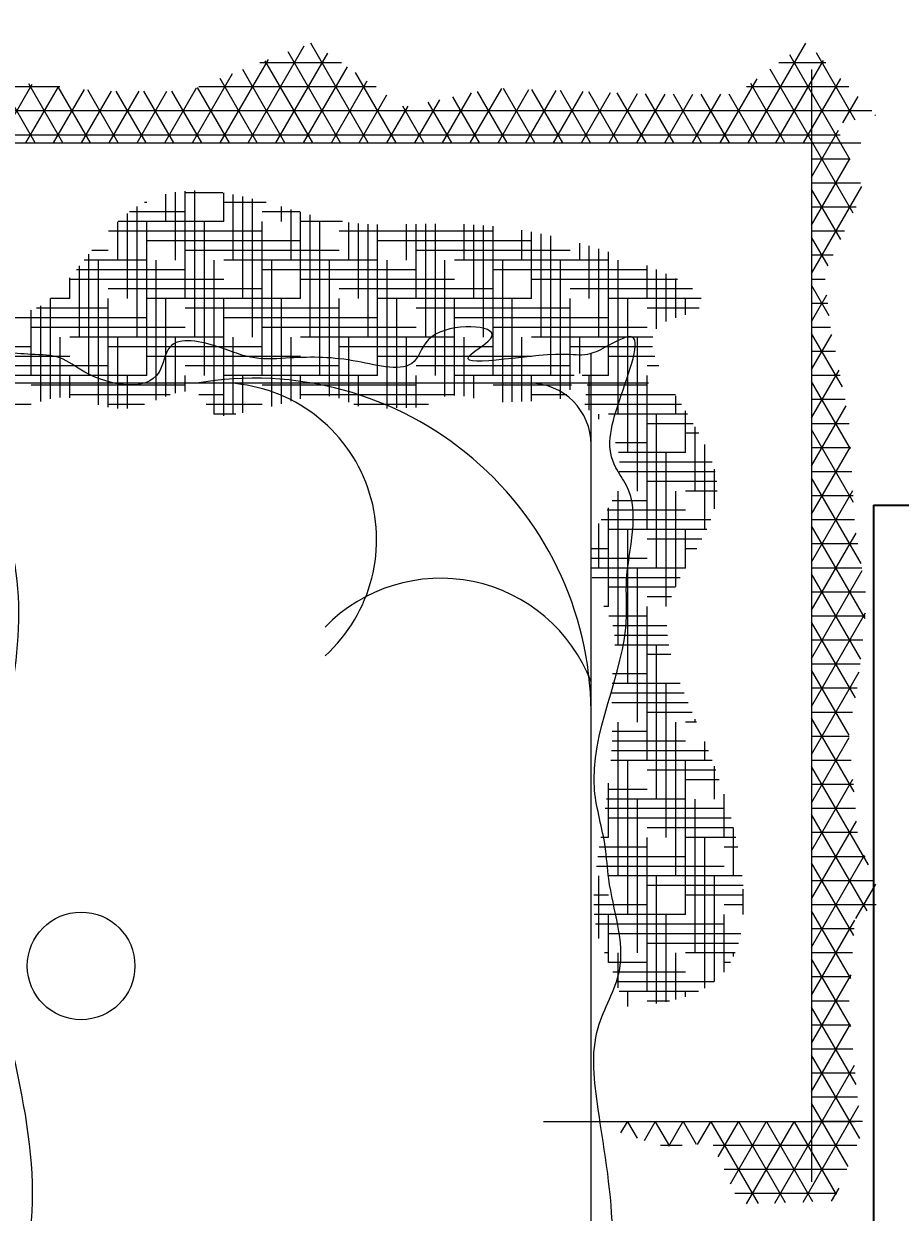
# Model space of a CAD drawing. Units: inches. Extents: x 3731 to 4318, y 1310 to 2388.
# Tile 6 of 57: x 3897 to 3944, y 1452 to 1515. Entities that reach past the tile are written whole.
import ezdxf

# ---------------------------------------------------------------- set-up
doc = ezdxf.new("R2010")
doc.units = ezdxf.units.IN
for name, color, linetype, lineweight in [('A-ANNO-DIMS', 2, 'Continuous', 18), ('A-FURN', 8, 'Continuous', 13), ('A-WALL', 7, 'Continuous', 35)]:
    doc.layers.add(name, color=color, linetype=linetype, lineweight=lineweight)
doc.styles.get("Standard").update_dxf_attribs({"font": 'arial.ttf'})
doc.dimstyles.get("Standard").update_dxf_attribs({"dimtxt": 0.18, "dimasz": 0.18, "dimexe": 0.18, "dimexo": 0.0625, "dimgap": 0.09, "dimtad": 0, "dimtih": 1, "dimtoh": 1, "dimdec": 4, "dimzin": 0, "dimdsep": 46, "dimtxsty": 'Standard', "dimcen": 0.09, "dimadec": 0, "dimazin": 0, "dimtfac": 1, "dimtdec": 4, "dimtofl": 0, "dimtmove": 0, "dimatfit": 3, "dimfxl": 1, "dimtolj": 1, "dimtzin": 0, "dimarcsym": 0})

# ---------------------------------------------------------------- blocks, each defined once
blk = doc.blocks.new('A$C200C7901')
for p, q in [((2.3121, 1.6596), (2.3121, 0.0201)), ((2, 0.2957), (2, 1.2957)), ((2.0224, 0.9977), (2.0224, 1.1977)), ((2.0224, 0.9977), (2.0224, 1.1977)), ((1.9974, 0.5977), (1.9974, 0.7977)), ((1.9974, 0.5977), (1.9974, 0.7977)), ((2.0724, 0.5977), (2.0724, 0.7977)), ((2.0724, 0.5977), (2.0724, 0.7977)), ((2.1474, 0.5977), (2.1474, 0.7977)), ((2.1474, 0.5977), (2.1474, 0.7977)), ((1.9849, 0.5477), (1.9849, 0.7477)), ((1.9849, 0.5477), (1.9849, 0.7477)), ((2.0599, 0.5477), (2.0599, 0.7477)), ((2.0599, 0.5477), (2.0599, 0.7477)), ((2.1349, 0.5477), (2.1349, 0.7477)), ((2.1349, 0.5477), (2.1349, 0.7477)), ((1.0407, 0.0275), (1.0407, 0.4323)), ((0.4061, 0.3703), (2.0386, 0.3703)), ((2.4073, 0.0839), (0.9625, 0.0839))]:
    blk.add_line(p, q)
at = {"linetype": 'ByBlock'}
for p, q in [((2.3224, 0.0468), (2.3224, 1.6627)), ((2.3224, 0.0468), (2.3224, 1.6627)), ((2.3537, 0.0056), (2.3537, 1.634)), ((2.3537, 0.0056), (2.3537, 1.634)), ((2.0474, 1.0977), (2.0474, 1.2977)), ((2.0474, 1.0977), (2.0474, 1.2977)), ((2.3849, 1.0607), (2.3849, 1.3013)), ((2.3849, 1.0607), (2.3849, 1.3013)), ((1.9724, 1.0977), (1.9724, 1.2927)), ((1.9724, 1.0977), (1.9724, 1.2927)), ((2.0349, 1.0477), (2.0349, 1.2477)), ((2.0349, 1.0477), (2.0349, 1.2477)), ((2.0099, 0.9477), (2.0099, 1.1477)), ((2.0099, 0.9477), (2.0099, 1.1477)), ((2.0849, 0.9477), (2.0849, 1.1477)), ((2.0849, 0.9477), (2.0849, 1.1477)), ((2.3121, 1.1408), (2.3884, 1.0967)), ((2.3121, 1.1408), (2.3884, 1.0967)), ((2.3121, 1.0928), (2.3915, 1.1386)), ((2.3121, 1.0928), (2.3915, 1.1386)), ((1.9974, 0.8977), (1.9974, 1.0977)), ((1.9974, 0.8977), (1.9974, 1.0977)), ((2.0099, 1.0977), (2.095, 1.0977)), ((2.0099, 1.0977), (2.095, 1.0977)), ((2.0724, 0.8977), (2.0724, 1.0977)), ((2.0724, 0.8977), (2.0724, 1.0977)), ((2.3121, 1.1047), (2.3851, 1.0625)), ((2.3121, 1.1047), (2.3851, 1.0625)), ((2.3121, 1.0567), (2.3887, 1.1009)), ((2.3121, 1.0567), (2.3887, 1.1009)), ((1.9763, 1.0852), (2.1005, 1.0852)), ((1.9763, 1.0852), (2.1005, 1.0852)), ((2.0974, 0.9977), (2.0974, 1.0909)), ((2.0974, 0.9977), (2.0974, 1.0909)), ((1.9799, 1.0727), (2.1099, 1.0727)), ((1.9799, 1.0727), (2.1099, 1.0727)), ((2.1099, 1.0477), (2.1099, 1.0729)), ((2.1099, 1.0477), (2.1099, 1.0729)), ((2.3121, 1.0686), (2.3813, 1.0286)), ((2.3121, 1.0686), (2.3813, 1.0286)), ((1.9815, 1.0602), (2.0599, 1.0602)), ((1.9815, 1.0602), (2.0599, 1.0602)), ((2.3121, 1.0206), (2.3851, 1.0628)), ((2.3121, 1.0206), (2.3851, 1.0628)), ((1.981, 1.0477), (2.0099, 1.0477)), ((1.981, 1.0477), (2.0099, 1.0477)), ((1.9849, 0.9171), (1.9849, 1.0477)), ((1.9849, 0.9171), (1.9849, 1.0477)), ((2.0599, 0.8477), (2.0599, 1.0477)), ((2.0599, 0.8477), (2.0599, 1.0477)), ((2.0599, 1.0352), (2.1523, 1.0352)), ((2.0599, 1.0352), (2.1523, 1.0352)), ((2.1099, 1.0477), (2.137, 1.0477)), ((2.1099, 1.0477), (2.137, 1.0477)), ((2.1349, 0.8477), (2.1349, 1.0477)), ((2.1349, 0.8477), (2.1349, 1.0477)), ((2.1474, 0.8977), (2.1474, 1.0391)), ((2.1474, 0.8977), (2.1474, 1.0391)), ((2.0099, 1.0227), (2.1678, 1.0227)), ((2.0099, 1.0227), (2.1678, 1.0227)), ((2.1599, 0.9477), (2.1599, 1.029)), ((2.1599, 0.9477), (2.1599, 1.029)), ((2.1724, 0.9977), (2.1724, 1.0189)), ((2.1724, 0.9977), (2.1724, 1.0189)), ((2.3121, 1.0325), (2.3795, 0.9936)), ((2.3121, 1.0325), (2.3795, 0.9936)), ((2.3121, 0.9846), (2.3809, 1.0242)), ((2.3121, 0.9846), (2.3809, 1.0242)), ((1.9718, 1.0102), (2.1599, 1.0102)), ((1.9718, 1.0102), (2.1599, 1.0102)), ((1.9688, 0.9977), (2.1099, 0.9977)), ((1.9688, 0.9977), (2.1099, 0.9977)), ((1.9724, 0.9504), (1.9724, 0.9977)), ((1.9724, 0.9504), (1.9724, 0.9977)), ((2.0474, 0.7977), (2.0474, 0.9977)), ((2.0474, 0.7977), (2.0474, 0.9977)), ((2.1224, 0.7977), (2.1224, 0.9977)), ((2.1224, 0.7977), (2.1224, 0.9977)), ((2.1974, 0.7977), (2.1974, 0.9972)), ((2.1974, 0.7977), (2.1974, 0.9972)), ((2.3121, 0.9964), (2.3795, 0.9575)), ((2.3121, 0.9964), (2.3795, 0.9575)), ((1.9671, 0.9852), (2.0599, 0.9852)), ((1.9671, 0.9852), (2.0599, 0.9852)), ((1.9672, 0.9727), (2.0099, 0.9727)), ((1.9672, 0.9727), (2.0099, 0.9727)), ((2.1099, 0.9727), (2.2204, 0.9727)), ((2.1099, 0.9727), (2.2204, 0.9727)), ((2.1599, 0.9852), (2.2095, 0.9852)), ((2.1599, 0.9852), (2.2095, 0.9852)), ((2.2099, 0.8477), (2.2099, 0.9848)), ((2.2099, 0.8477), (2.2099, 0.9848)), ((2.3121, 0.9485), (2.3795, 0.9874)), ((2.3121, 0.9485), (2.3795, 0.9874)), ((2.0599, 0.9602), (2.2294, 0.9602)), ((2.0599, 0.9602), (2.2294, 0.9602)), ((2.2224, 0.8977), (2.2224, 0.9702)), ((2.2224, 0.8977), (2.2224, 0.9702)), ((2.3121, 0.9603), (2.3795, 0.9215)), ((2.3121, 0.9603), (2.3795, 0.9215)), ((2.0099, 0.9477), (2.2099, 0.9477)), ((2.0099, 0.9477), (2.2099, 0.9477)), ((2.0349, 0.7477), (2.0349, 0.9477)), ((2.0349, 0.7477), (2.0349, 0.9477)), ((2.1099, 0.7477), (2.1099, 0.9477)), ((2.1099, 0.7477), (2.1099, 0.9477)), ((2.1849, 0.7477), (2.1849, 0.9477)), ((2.1849, 0.7477), (2.1849, 0.9477)), ((2.2349, 0.9477), (2.2349, 0.9506)), ((2.2349, 0.9477), (2.2349, 0.9506)), ((2.3121, 0.9124), (2.3795, 0.9513)), ((2.3121, 0.9124), (2.3795, 0.9513)), ((1.9781, 0.9352), (2.1599, 0.9352)), ((1.9781, 0.9352), (2.1599, 0.9352)), ((1.9829, 0.9227), (2.1099, 0.9227)), ((1.9829, 0.9227), (2.1099, 0.9227)), ((2.2099, 0.9227), (2.2455, 0.9227)), ((2.2099, 0.9227), (2.2455, 0.9227)), ((2.3121, 0.9243), (2.3838, 0.8829)), ((2.3121, 0.9243), (2.3838, 0.8829)), ((2.3121, 0.8763), (2.3795, 0.9152)), ((2.3121, 0.8763), (2.3795, 0.9152)), ((1.9871, 0.9102), (2.0599, 0.9102)), ((1.9871, 0.9102), (2.0599, 0.9102)), ((1.9894, 0.8977), (2.0099, 0.8977)), ((1.9894, 0.8977), (2.0099, 0.8977)), ((2.0224, 0.6977), (2.0224, 0.8977)), ((2.0224, 0.6977), (2.0224, 0.8977)), ((2.0974, 0.6977), (2.0974, 0.8977)), ((2.0974, 0.6977), (2.0974, 0.8977)), ((2.1099, 0.8977), (2.2496, 0.8977)), ((2.1099, 0.8977), (2.2496, 0.8977)), ((2.1599, 0.9102), (2.2481, 0.9102)), ((2.1599, 0.9102), (2.2481, 0.9102)), ((2.1724, 0.6977), (2.1724, 0.8977)), ((2.1724, 0.6977), (2.1724, 0.8977)), ((2.2474, 0.8489), (2.2474, 0.8977)), ((2.2474, 0.8489), (2.2474, 0.8977)), ((1.9849, 0.8477), (1.9849, 0.88)), ((1.9849, 0.8477), (1.9849, 0.88)), ((2.0599, 0.8852), (2.2501, 0.8852)), ((2.0599, 0.8852), (2.2501, 0.8852)), ((2.3121, 0.8882), (2.4022, 0.8362)), ((2.3121, 0.8882), (2.4022, 0.8362)), ((2.3121, 0.8402), (2.3842, 0.8818)), ((2.3121, 0.8402), (2.3842, 0.8818)), ((2.3849, 0.6497), (2.3849, 0.8801)), ((2.3849, 0.6497), (2.3849, 0.8801)), ((1.9724, 0.7977), (1.9724, 0.8703)), ((1.9724, 0.7977), (1.9724, 0.8703)), ((2.0099, 0.8727), (2.2099, 0.8727)), ((2.0099, 0.8727), (2.2099, 0.8727)), ((1.9599, 0.8317), (1.9599, 0.8604)), ((1.9599, 0.8317), (1.9599, 0.8604)), ((1.9599, 0.8602), (2.1599, 0.8602)), ((1.9599, 0.8602), (2.1599, 0.8602)), ((2.3121, 0.8041), (2.3958, 0.8524)), ((2.3121, 0.8041), (2.3958, 0.8524)), ((2.3121, 0.8521), (2.4205, 0.7895)), ((2.3121, 0.8521), (2.4205, 0.7895)), ((1.9574, 0.8477), (2.1099, 0.8477)), ((1.9574, 0.8477), (2.1099, 0.8477)), ((1.9593, 0.8352), (2.0599, 0.8352)), ((1.9593, 0.8352), (2.0599, 0.8352)), ((2.0099, 0.6477), (2.0099, 0.8477)), ((2.0099, 0.6477), (2.0099, 0.8477)), ((2.0849, 0.6477), (2.0849, 0.8477)), ((2.0849, 0.6477), (2.0849, 0.8477)), ((2.1599, 0.6477), (2.1599, 0.8477)), ((2.1599, 0.6477), (2.1599, 0.8477)), ((2.1599, 0.8352), (2.2451, 0.8352)), ((2.1599, 0.8352), (2.2451, 0.8352)), ((2.2099, 0.8477), (2.2472, 0.8477)), ((2.2099, 0.8477), (2.2472, 0.8477)), ((2.2349, 0.7923), (2.2349, 0.8477)), ((2.2349, 0.7923), (2.2349, 0.8477)), ((1.9615, 0.8227), (2.0099, 0.8227)), ((1.9615, 0.8227), (2.0099, 0.8227)), ((2.1099, 0.8227), (2.2425, 0.8227)), ((2.1099, 0.8227), (2.2425, 0.8227)), ((2.3121, 0.7681), (2.4073, 0.823)), ((2.3121, 0.7681), (2.4073, 0.823)), ((2.0599, 0.8102), (2.2396, 0.8102)), ((2.0599, 0.8102), (2.2396, 0.8102)), ((2.3121, 0.816), (2.4384, 0.7431)), ((2.3121, 0.816), (2.4384, 0.7431)), ((2.0099, 0.7977), (2.2099, 0.7977)), ((2.0099, 0.7977), (2.2099, 0.7977)), ((2.2224, 0.7483), (2.2224, 0.7977)), ((2.2224, 0.7483), (2.2224, 0.7977)), ((2.3121, 0.732), (2.4189, 0.7936)), ((2.3121, 0.732), (2.4189, 0.7936)), ((2.4162, 0.6946), (2.4162, 0.8006)), ((2.4162, 0.6946), (2.4162, 0.8006)), ((1.9699, 0.7852), (2.1599, 0.7852)), ((1.9699, 0.7852), (2.1599, 0.7852)), ((1.9734, 0.7727), (2.1099, 0.7727)), ((1.9734, 0.7727), (2.1099, 0.7727)), ((2.2099, 0.7727), (2.2294, 0.7727)), ((2.2099, 0.7727), (2.2294, 0.7727)), ((2.3121, 0.7799), (2.4287, 0.7126)), ((2.3121, 0.7799), (2.4287, 0.7126)), ((1.9767, 0.7602), (2.0599, 0.7602)), ((1.9767, 0.7602), (2.0599, 0.7602)), ((2.1599, 0.7602), (2.2258, 0.7602)), ((2.1599, 0.7602), (2.2258, 0.7602)), ((2.3121, 0.6959), (2.4303, 0.7641)), ((2.3121, 0.6959), (2.4303, 0.7641)), ((1.9797, 0.7477), (2.0099, 0.7477)), ((1.9797, 0.7477), (2.0099, 0.7477)), ((2.1099, 0.7477), (2.2222, 0.7477)), ((2.1099, 0.7477), (2.2222, 0.7477)), ((2.2099, 0.6933), (2.2099, 0.7477)), ((2.2099, 0.6933), (2.2099, 0.7477)), ((2.3121, 0.7438), (2.4108, 0.6869)), ((2.3121, 0.7438), (2.4108, 0.6869)), ((2.0599, 0.7352), (2.2188, 0.7352)), ((2.0599, 0.7352), (2.2188, 0.7352)), ((2.3121, 0.6598), (2.4417, 0.7346)), ((2.3121, 0.6598), (2.4417, 0.7346)), ((1.9831, 0.7102), (2.1599, 0.7102)), ((1.9831, 0.7102), (2.1599, 0.7102)), ((2.0099, 0.7227), (2.2099, 0.7227)), ((2.0099, 0.7227), (2.2099, 0.7227)), ((1.9804, 0.6977), (2.1099, 0.6977)), ((1.9804, 0.6977), (2.1099, 0.6977)), ((2.0474, 0.4977), (2.0474, 0.6977)), ((2.0474, 0.4977), (2.0474, 0.6977)), ((2.1224, 0.4977), (2.1224, 0.6977)), ((2.1224, 0.4977), (2.1224, 0.6977)), ((2.1974, 0.4977), (2.1974, 0.6977)), ((2.1974, 0.4977), (2.1974, 0.6977)), ((2.2099, 0.6977), (2.2106, 0.6977)), ((2.2099, 0.6977), (2.2106, 0.6977)), ((2.3121, 0.7078), (2.3929, 0.6611)), ((2.3121, 0.7078), (2.3929, 0.6611)), ((1.9753, 0.6852), (2.0599, 0.6852)), ((1.9753, 0.6852), (2.0599, 0.6852)), ((2.1599, 0.6852), (2.2088, 0.6852)), ((2.1599, 0.6852), (2.2088, 0.6852)), ((1.97, 0.6727), (2.0099, 0.6727)), ((1.97, 0.6727), (2.0099, 0.6727)), ((1.9724, 0.5818), (1.9724, 0.6786)), ((1.9724, 0.5818), (1.9724, 0.6786)), ((2.1099, 0.6727), (2.2075, 0.6727)), ((2.1099, 0.6727), (2.2075, 0.6727)), ((2.3121, 0.6237), (2.4036, 0.6765)), ((2.3121, 0.6237), (2.4036, 0.6765)), ((2.3121, 0.6717), (2.3744, 0.6357)), ((2.3121, 0.6717), (2.3744, 0.6357)), ((2.0599, 0.6602), (2.2067, 0.6602)), ((2.0599, 0.6602), (2.2067, 0.6602)), ((1.9673, 0.6352), (2.1599, 0.6352)), ((1.9673, 0.6352), (2.1599, 0.6352)), ((2.0099, 0.6477), (2.2062, 0.6477)), ((2.0099, 0.6477), (2.2062, 0.6477)), ((2.0349, 0.4477), (2.0349, 0.6477)), ((2.0349, 0.4477), (2.0349, 0.6477)), ((2.1099, 0.4477), (2.1099, 0.6477)), ((2.1099, 0.4477), (2.1099, 0.6477)), ((2.1849, 0.4477), (2.1849, 0.6477)), ((2.1849, 0.4477), (2.1849, 0.6477)), ((2.3121, 0.6356), (2.3598, 0.6081)), ((2.3121, 0.6356), (2.3598, 0.6081)), ((1.9678, 0.6227), (2.1099, 0.6227)), ((1.9678, 0.6227), (2.1099, 0.6227)), ((1.9679, 0.6102), (2.0599, 0.6102)), ((1.9679, 0.6102), (2.0599, 0.6102)), ((2.1599, 0.6102), (2.2064, 0.6102)), ((2.1599, 0.6102), (2.2064, 0.6102)), ((2.3121, 0.5876), (2.3598, 0.6151)), ((2.3121, 0.5876), (2.3598, 0.6151)), ((1.9685, 0.5977), (2.0099, 0.5977)), ((1.9685, 0.5977), (2.0099, 0.5977)), ((2.0224, 0.3977), (2.0224, 0.5977)), ((2.0224, 0.3977), (2.0224, 0.5977)), ((2.0974, 0.3977), (2.0974, 0.5977)), ((2.0974, 0.3977), (2.0974, 0.5977)), ((2.1099, 0.5977), (2.2066, 0.5977)), ((2.1099, 0.5977), (2.2066, 0.5977)), ((2.1724, 0.3977), (2.1724, 0.5977)), ((2.1724, 0.3977), (2.1724, 0.5977)), ((2.3121, 0.5995), (2.3682, 0.5671)), ((2.3121, 0.5995), (2.3682, 0.5671)), ((2.0099, 0.5727), (2.207, 0.5727)), ((2.0099, 0.5727), (2.207, 0.5727)), ((2.0599, 0.5852), (2.2069, 0.5852)), ((2.0599, 0.5852), (2.2069, 0.5852)), ((2.3121, 0.5515), (2.365, 0.5821)), ((2.3121, 0.5515), (2.365, 0.5821)), ((1.9827, 0.5602), (2.1599, 0.5602)), ((1.9827, 0.5602), (2.1599, 0.5602)), ((2.3121, 0.5634), (2.3771, 0.5259)), ((2.3121, 0.5634), (2.3771, 0.5259)), ((1.9842, 0.5477), (2.1099, 0.5477)), ((1.9842, 0.5477), (2.1099, 0.5477)), ((2.0099, 0.3923), (2.0099, 0.5477)), ((2.0099, 0.3923), (2.0099, 0.5477)), ((2.0849, 0.3477), (2.0849, 0.5477)), ((2.0849, 0.3477), (2.0849, 0.5477)), ((2.1599, 0.3477), (2.1599, 0.5477)), ((2.1599, 0.3477), (2.1599, 0.5477)), ((2.3121, 0.5155), (2.3719, 0.55)), ((2.3121, 0.5155), (2.3719, 0.55)), ((1.9831, 0.5352), (2.0599, 0.5352)), ((1.9831, 0.5352), (2.0599, 0.5352)), ((2.1599, 0.5352), (2.2065, 0.5352)), ((2.1599, 0.5352), (2.2065, 0.5352)), ((2.3121, 0.5273), (2.383, 0.4864)), ((2.3121, 0.5273), (2.383, 0.4864)), ((1.9807, 0.5227), (2.0099, 0.5227)), ((1.9807, 0.5227), (2.0099, 0.5227)), ((2.0599, 0.5102), (2.2049, 0.5102)), ((2.0599, 0.5102), (2.2049, 0.5102)), ((2.1099, 0.5227), (2.2058, 0.5227)), ((2.1099, 0.5227), (2.2058, 0.5227)), ((2.3121, 0.4794), (2.3788, 0.5179)), ((2.3121, 0.4794), (2.3788, 0.5179)), ((1.9974, 0.3957), (1.9974, 0.4977)), ((1.9974, 0.3957), (1.9974, 0.4977)), ((2.0099, 0.4977), (2.2038, 0.4977)), ((2.0099, 0.4977), (2.2038, 0.4977)), ((2.0724, 0.2977), (2.0724, 0.4977)), ((2.0724, 0.2977), (2.0724, 0.4977)), ((2.1474, 0.2977), (2.1474, 0.4977)), ((2.1474, 0.2977), (2.1474, 0.4977)), ((1.9755, 0.4852), (2.1599, 0.4852)), ((1.9755, 0.4852), (2.1599, 0.4852)), ((2.3121, 0.4912), (2.3817, 0.4511)), ((2.3121, 0.4912), (2.3817, 0.4511)), ((2.3121, 0.4433), (2.383, 0.4842)), ((2.3121, 0.4433), (2.383, 0.4842)), ((1.9757, 0.4727), (2.1099, 0.4727)), ((1.9757, 0.4727), (2.1099, 0.4727)), ((1.9762, 0.4602), (2.0599, 0.4602)), ((1.9762, 0.4602), (2.0599, 0.4602)), ((2.1599, 0.4602), (2.1987, 0.4602)), ((2.1599, 0.4602), (2.1987, 0.4602)), ((2.3121, 0.4552), (2.3803, 0.4158)), ((2.3121, 0.4552), (2.3803, 0.4158)), ((1.9768, 0.4477), (2.0099, 0.4477)), ((1.9768, 0.4477), (2.0099, 0.4477)), ((1.9849, 0.402), (1.9849, 0.4477)), ((1.9849, 0.402), (1.9849, 0.4477)), ((2.0599, 0.2903), (2.0599, 0.4477)), ((2.0599, 0.2903), (2.0599, 0.4477)), ((2.0599, 0.4352), (2.194, 0.4352)), ((2.0599, 0.4352), (2.194, 0.4352)), ((2.1099, 0.4477), (2.1965, 0.4477)), ((2.1099, 0.4477), (2.1965, 0.4477)), ((2.1349, 0.2582), (2.1349, 0.4477)), ((2.1349, 0.2582), (2.1349, 0.4477)), ((2.3121, 0.4072), (2.3815, 0.4473)), ((2.3121, 0.4072), (2.3815, 0.4473)), ((2.0099, 0.4227), (2.1913, 0.4227)), ((2.0099, 0.4227), (2.1913, 0.4227)), ((2.3121, 0.4191), (2.3789, 0.3805)), ((2.3121, 0.4191), (2.3789, 0.3805)), ((1.9797, 0.4102), (2.1599, 0.4102)), ((1.9797, 0.4102), (2.1599, 0.4102)), ((2.3121, 0.3711), (2.3801, 0.4103)), ((2.3121, 0.3711), (2.3801, 0.4103)), ((1.9915, 0.3977), (2.1099, 0.3977)), ((1.9915, 0.3977), (2.1099, 0.3977)), ((2.0474, 0.2905), (2.0474, 0.3977)), ((2.0474, 0.2905), (2.0474, 0.3977)), ((2.1224, 0.2385), (2.1224, 0.3977)), ((2.1224, 0.2385), (2.1224, 0.3977)), ((1.9648, 0.3727), (2.0099, 0.3727)), ((1.9648, 0.3727), (2.0099, 0.3727)), ((1.9724, 0.253), (1.9724, 0.3785)), ((1.9724, 0.253), (1.9724, 0.3785)), ((1.9849, 0.2609), (1.9849, 0.3774)), ((1.9849, 0.2609), (1.9849, 0.3774)), ((1.9974, 0.2977), (1.9974, 0.3753)), ((1.9974, 0.2977), (1.9974, 0.3753)), ((2.0099, 0.3477), (2.0099, 0.382)), ((2.0099, 0.3477), (2.0099, 0.382)), ((2.0127, 0.3852), (2.0599, 0.3852)), ((2.0127, 0.3852), (2.0599, 0.3852)), ((2.1099, 0.3727), (2.1784, 0.3727)), ((2.1099, 0.3727), (2.1784, 0.3727)), ((2.1599, 0.3852), (2.1819, 0.3852)), ((2.1599, 0.3852), (2.1819, 0.3852)), ((2.3121, 0.383), (2.3775, 0.3452)), ((2.3121, 0.383), (2.3775, 0.3452)), ((2.3121, 0.335), (2.3786, 0.3734)), ((2.3121, 0.335), (2.3786, 0.3734)), ((1.2785, 0.3602), (1.3599, 0.3602)), ((1.2785, 0.3602), (1.3599, 0.3602)), ((1.2974, 0.1977), (1.2974, 0.3647)), ((1.2974, 0.1977), (1.2974, 0.3647)), ((1.3099, 0.2477), (1.3099, 0.3663)), ((1.3099, 0.2477), (1.3099, 0.3663)), ((1.3224, 0.2977), (1.3224, 0.3669)), ((1.3224, 0.2977), (1.3224, 0.3669)), ((1.3349, 0.3477), (1.3349, 0.3668)), ((1.3349, 0.3477), (1.3349, 0.3668)), ((1.3724, 0.1977), (1.3724, 0.3634)), ((1.3724, 0.1977), (1.3724, 0.3634)), ((1.3849, 0.2477), (1.3849, 0.3616)), ((1.3849, 0.2477), (1.3849, 0.3616)), ((1.3974, 0.2977), (1.3974, 0.3597)), ((1.3974, 0.2977), (1.3974, 0.3597)), ((1.4099, 0.3477), (1.4099, 0.3578)), ((1.4099, 0.3477), (1.4099, 0.3578)), ((1.7474, 0.2546), (1.7474, 0.3689)), ((1.7474, 0.2546), (1.7474, 0.3689)), ((1.7599, 0.2477), (1.7599, 0.3703)), ((1.7599, 0.2477), (1.7599, 0.3703)), ((1.7599, 0.3602), (1.8177, 0.3602)), ((1.7599, 0.3602), (1.8177, 0.3602)), ((1.7724, 0.2977), (1.7724, 0.3703)), ((1.7724, 0.2977), (1.7724, 0.3703)), ((1.7849, 0.3477), (1.7849, 0.3703)), ((1.7849, 0.3477), (1.7849, 0.3703)), ((1.8224, 0.2148), (1.8224, 0.3575)), ((1.8224, 0.2148), (1.8224, 0.3575)), ((1.9532, 0.3602), (1.9599, 0.3602)), ((1.9532, 0.3602), (1.9599, 0.3602)), ((2.0599, 0.3602), (2.1747, 0.3602)), ((2.0599, 0.3602), (2.1747, 0.3602)), ((1.2349, 0.2477), (1.2349, 0.3422)), ((1.2349, 0.2477), (1.2349, 0.3422)), ((1.2474, 0.2977), (1.2474, 0.3476)), ((1.2474, 0.2977), (1.2474, 0.3476)), ((1.2475, 0.3477), (1.3099, 0.3477)), ((1.2475, 0.3477), (1.3099, 0.3477)), ((1.2599, 0.3477), (1.2599, 0.3531)), ((1.2599, 0.3477), (1.2599, 0.3531)), ((1.2849, 0.1758), (1.2849, 0.3477)), ((1.2849, 0.1758), (1.2849, 0.3477)), ((1.3599, 0.1741), (1.3599, 0.3477)), ((1.3599, 0.1741), (1.3599, 0.3477)), ((1.4099, 0.3477), (1.4806, 0.3477)), ((1.4099, 0.3477), (1.4806, 0.3477)), ((1.4349, 0.1886), (1.4349, 0.3477)), ((1.4349, 0.1886), (1.4349, 0.3477)), ((1.4474, 0.1977), (1.4474, 0.3521)), ((1.4474, 0.1977), (1.4474, 0.3521)), ((1.4599, 0.2477), (1.4599, 0.3504)), ((1.4599, 0.2477), (1.4599, 0.3504)), ((1.4724, 0.2977), (1.4724, 0.3487)), ((1.4724, 0.2977), (1.4724, 0.3487)), ((1.5099, 0.2129), (1.5099, 0.3447)), ((1.5099, 0.2129), (1.5099, 0.3447)), ((1.5224, 0.2177), (1.5224, 0.3438)), ((1.5224, 0.2177), (1.5224, 0.3438)), ((1.5349, 0.2477), (1.5349, 0.3431)), ((1.5349, 0.2477), (1.5349, 0.3431)), ((1.5474, 0.2977), (1.5474, 0.3428)), ((1.5474, 0.2977), (1.5474, 0.3428)), ((1.5849, 0.2443), (1.5849, 0.3434)), ((1.5849, 0.2443), (1.5849, 0.3434)), ((1.5974, 0.2496), (1.5974, 0.3435)), ((1.5974, 0.2496), (1.5974, 0.3435)), ((1.6099, 0.2546), (1.6099, 0.3432)), ((1.6099, 0.2546), (1.6099, 0.3432)), ((1.6224, 0.2977), (1.6224, 0.3424)), ((1.6224, 0.2977), (1.6224, 0.3424)), ((1.6724, 0.2713), (1.6724, 0.3398)), ((1.6724, 0.2713), (1.6724, 0.3398)), ((1.6849, 0.272), (1.6849, 0.3422)), ((1.6849, 0.272), (1.6849, 0.3422)), ((1.6974, 0.2977), (1.6974, 0.3472)), ((1.6974, 0.2977), (1.6974, 0.3472)), ((1.7099, 0.3477), (1.7099, 0.3539)), ((1.7099, 0.3477), (1.7099, 0.3539)), ((1.7099, 0.3477), (1.8383, 0.3477)), ((1.7099, 0.3477), (1.8383, 0.3477)), ((1.7349, 0.2607), (1.7349, 0.3477)), ((1.7349, 0.2607), (1.7349, 0.3477)), ((1.8099, 0.2201), (1.8099, 0.3477)), ((1.8099, 0.2201), (1.8099, 0.3477)), ((1.8349, 0.2477), (1.8349, 0.3497)), ((1.8349, 0.2477), (1.8349, 0.3497)), ((1.8474, 0.2977), (1.8474, 0.3432)), ((1.8474, 0.2977), (1.8474, 0.3432)), ((1.9599, 0.2452), (1.9599, 0.3477)), ((1.9599, 0.2452), (1.9599, 0.3477)), ((2.0099, 0.3477), (2.1708, 0.3477)), ((2.0099, 0.3477), (2.1708, 0.3477)), ((2.0349, 0.2874), (2.0349, 0.3477)), ((2.0349, 0.2874), (2.0349, 0.3477)), ((2.1099, 0.2274), (2.1099, 0.3477)), ((2.1099, 0.2274), (2.1099, 0.3477)), ((2.3121, 0.3469), (2.3761, 0.31)), ((2.3121, 0.3469), (2.3761, 0.31)), ((1.0261, 0.3316), (1.0407, 0.3232)), ((1.0261, 0.3316), (1.0407, 0.3232)), ((1.2099, 0.2308), (1.2099, 0.334)), ((1.2099, 0.2308), (1.2099, 0.334)), ((1.2148, 0.3352), (1.2599, 0.3352)), ((1.2148, 0.3352), (1.2599, 0.3352)), ((1.2224, 0.2106), (1.2224, 0.3375)), ((1.2224, 0.2106), (1.2224, 0.3375)), ((1.3599, 0.3352), (1.5599, 0.3352)), ((1.3599, 0.3352), (1.5599, 0.3352)), ((1.6599, 0.2695), (1.6599, 0.3394)), ((1.6599, 0.2695), (1.6599, 0.3394)), ((1.6599, 0.3352), (1.8599, 0.3352)), ((1.6599, 0.3352), (1.8599, 0.3352)), ((1.8849, 0.2093), (1.8849, 0.3337)), ((1.8849, 0.2093), (1.8849, 0.3337)), ((1.8974, 0.2129), (1.8974, 0.3335)), ((1.8974, 0.2129), (1.8974, 0.3335)), ((1.9099, 0.2477), (1.9099, 0.3349)), ((1.9099, 0.2477), (1.9099, 0.3349)), ((1.9224, 0.2977), (1.9224, 0.3385)), ((1.9224, 0.2977), (1.9224, 0.3385)), ((1.9599, 0.3352), (2.1599, 0.3352)), ((1.9599, 0.3352), (2.1599, 0.3352)), ((2.3121, 0.299), (2.3772, 0.3365)), ((2.3121, 0.299), (2.3772, 0.3365)), ((1.0194, 0.3103), (1.0407, 0.3227)), ((1.0194, 0.3103), (1.0407, 0.3227)), ((1.1904, 0.3227), (1.2099, 0.3227)), ((1.1904, 0.3227), (1.2099, 0.3227)), ((1.2599, 0.3102), (1.4599, 0.3102)), ((1.2599, 0.3102), (1.4599, 0.3102)), ((1.3099, 0.3227), (1.5099, 0.3227)), ((1.3099, 0.3227), (1.5099, 0.3227)), ((1.5599, 0.3102), (1.7599, 0.3102)), ((1.5599, 0.3102), (1.7599, 0.3102)), ((1.6099, 0.3227), (1.8099, 0.3227)), ((1.6099, 0.3227), (1.8099, 0.3227)), ((1.8599, 0.3102), (2.0599, 0.3102)), ((1.8599, 0.3102), (2.0599, 0.3102)), ((1.9099, 0.3227), (2.1099, 0.3227)), ((1.9099, 0.3227), (2.1099, 0.3227)), ((2.3121, 0.3108), (2.3755, 0.2742)), ((2.3121, 0.3108), (2.3755, 0.2742)), ((1.0164, 0.3011), (1.0407, 0.2871)), ((1.0164, 0.3011), (1.0407, 0.2871)), ((1.1974, 0.2683), (1.1974, 0.2977)), ((1.1974, 0.2683), (1.1974, 0.2977)), ((1.2099, 0.2977), (1.4099, 0.2977)), ((1.2099, 0.2977), (1.4099, 0.2977)), ((1.2724, 0.1788), (1.2724, 0.2977)), ((1.2724, 0.1788), (1.2724, 0.2977)), ((1.3474, 0.173), (1.3474, 0.2977)), ((1.3474, 0.173), (1.3474, 0.2977)), ((1.4224, 0.1854), (1.4224, 0.2977)), ((1.4224, 0.1854), (1.4224, 0.2977)), ((1.4974, 0.2083), (1.4974, 0.2977)), ((1.4974, 0.2083), (1.4974, 0.2977)), ((1.5099, 0.2977), (1.7099, 0.2977)), ((1.5099, 0.2977), (1.7099, 0.2977)), ((1.5724, 0.2389), (1.5724, 0.2977)), ((1.5724, 0.2389), (1.5724, 0.2977)), ((1.6474, 0.2668), (1.6474, 0.2977)), ((1.6474, 0.2668), (1.6474, 0.2977)), ((1.7224, 0.2658), (1.7224, 0.2977)), ((1.7224, 0.2658), (1.7224, 0.2977)), ((1.7974, 0.2263), (1.7974, 0.2977)), ((1.7974, 0.2263), (1.7974, 0.2977)), ((1.8099, 0.2977), (2.0099, 0.2977)), ((1.8099, 0.2977), (2.0099, 0.2977)), ((1.8724, 0.2072), (1.8724, 0.2977)), ((1.8724, 0.2072), (1.8724, 0.2977)), ((1.9474, 0.2376), (1.9474, 0.2977)), ((1.9474, 0.2376), (1.9474, 0.2977)), ((2.0224, 0.2822), (2.0224, 0.2977)), ((2.0224, 0.2822), (2.0224, 0.2977)), ((2.0974, 0.2299), (2.0974, 0.2977)), ((2.0974, 0.2299), (2.0974, 0.2977)), ((2.1099, 0.2977), (2.153, 0.2977)), ((2.1099, 0.2977), (2.153, 0.2977)), ((2.3121, 0.2629), (2.3757, 0.2996)), ((2.3121, 0.2629), (2.3757, 0.2996)), ((1.0089, 0.2682), (1.0407, 0.2866)), ((1.0089, 0.2682), (1.0407, 0.2866)), ((1.0099, 0.2521), (1.0099, 0.2804)), ((1.0099, 0.2521), (1.0099, 0.2804)), ((1.1943, 0.2852), (1.3599, 0.2852)), ((1.1943, 0.2852), (1.3599, 0.2852)), ((1.4599, 0.2852), (1.6599, 0.2852)), ((1.4599, 0.2852), (1.6599, 0.2852)), ((1.7599, 0.2852), (1.9599, 0.2852)), ((1.7599, 0.2852), (1.9599, 0.2852)), ((2.0708, 0.2852), (2.1478, 0.2852)), ((2.0708, 0.2852), (2.1478, 0.2852)), ((1.0088, 0.2694), (1.0407, 0.251)), ((1.0088, 0.2694), (1.0407, 0.251)), ((1.1965, 0.2727), (1.3099, 0.2727)), ((1.1965, 0.2727), (1.3099, 0.2727)), ((1.4099, 0.2727), (1.6099, 0.2727)), ((1.4099, 0.2727), (1.6099, 0.2727)), ((1.7099, 0.2727), (1.9099, 0.2727)), ((1.7099, 0.2727), (1.9099, 0.2727)), ((2.08, 0.2727), (2.1422, 0.2727)), ((2.08, 0.2727), (2.1422, 0.2727)), ((2.3121, 0.2747), (2.3755, 0.2381)), ((2.3121, 0.2747), (2.3755, 0.2381)), ((2.3121, 0.2268), (2.3755, 0.2634)), ((2.3121, 0.2268), (2.3755, 0.2634)), ((1.0111, 0.2334), (1.0407, 0.2505)), ((1.0111, 0.2334), (1.0407, 0.2505)), ((1.1994, 0.2602), (1.2599, 0.2602)), ((1.1994, 0.2602), (1.2599, 0.2602)), ((1.2031, 0.2477), (1.2099, 0.2477)), ((1.2031, 0.2477), (1.2099, 0.2477)), ((1.2599, 0.1831), (1.2599, 0.2477)), ((1.2599, 0.1831), (1.2599, 0.2477)), ((1.3099, 0.2477), (1.5099, 0.2477)), ((1.3099, 0.2477), (1.5099, 0.2477)), ((1.3349, 0.1723), (1.3349, 0.2477)), ((1.3349, 0.1723), (1.3349, 0.2477)), ((1.3599, 0.2602), (1.5599, 0.2602)), ((1.3599, 0.2602), (1.5599, 0.2602)), ((1.4099, 0.1825), (1.4099, 0.2477)), ((1.4099, 0.1825), (1.4099, 0.2477)), ((1.4849, 0.2039), (1.4849, 0.2477)), ((1.4849, 0.2039), (1.4849, 0.2477)), ((1.5599, 0.2335), (1.5599, 0.2477)), ((1.5599, 0.2335), (1.5599, 0.2477)), ((1.7361, 0.2602), (1.8599, 0.2602)), ((1.7361, 0.2602), (1.8599, 0.2602)), ((1.7599, 0.2477), (1.8099, 0.2477)), ((1.7599, 0.2477), (1.8099, 0.2477)), ((1.7849, 0.2332), (1.7849, 0.2477)), ((1.7849, 0.2332), (1.7849, 0.2477)), ((1.8599, 0.2068), (1.8599, 0.2477)), ((1.8599, 0.2068), (1.8599, 0.2477)), ((1.9099, 0.2477), (1.9639, 0.2477)), ((1.9099, 0.2477), (1.9639, 0.2477)), ((1.9349, 0.2304), (1.9349, 0.2477)), ((1.9349, 0.2304), (1.9349, 0.2477)), ((1.9599, 0.2602), (1.9838, 0.2602)), ((1.9599, 0.2602), (1.9838, 0.2602)), ((2.0848, 0.2602), (2.1359, 0.2602)), ((2.0848, 0.2602), (2.1359, 0.2602)), ((2.0888, 0.2477), (2.1099, 0.2477)), ((2.0888, 0.2477), (2.1099, 0.2477)), ((1.0112, 0.232), (1.0407, 0.215)), ((1.0112, 0.232), (1.0407, 0.215)), ((1.2599, 0.2352), (1.4599, 0.2352)), ((1.2599, 0.2352), (1.4599, 0.2352)), ((1.5599, 0.2352), (1.5638, 0.2352)), ((1.5599, 0.2352), (1.5638, 0.2352)), ((1.8599, 0.2352), (1.9433, 0.2352)), ((1.8599, 0.2352), (1.9433, 0.2352)), ((2.3121, 0.2387), (2.3755, 0.202)), ((2.3121, 0.2387), (2.3755, 0.202)), ((1.2142, 0.2227), (1.4099, 0.2227)), ((1.2142, 0.2227), (1.4099, 0.2227)), ((1.5099, 0.2227), (1.5346, 0.2227)), ((1.5099, 0.2227), (1.5346, 0.2227)), ((1.8099, 0.2227), (1.9203, 0.2227)), ((1.8099, 0.2227), (1.9203, 0.2227)), ((2.3121, 0.1907), (2.3755, 0.2273)), ((2.3121, 0.1907), (2.3755, 0.2273)), ((0.9344, 0.153), (1.0407, 0.2144)), ((0.9344, 0.153), (1.0407, 0.2144)), ((0.9953, 0.2051), (1.0407, 0.1789)), ((0.9953, 0.2051), (1.0407, 0.1789)), ((1.0099, 0.0251), (1.0099, 0.2117)), ((1.0099, 0.0251), (1.0099, 0.2117)), ((1.2227, 0.2102), (1.3599, 0.2102)), ((1.2227, 0.2102), (1.3599, 0.2102)), ((1.4599, 0.2102), (1.5027, 0.2102)), ((1.4599, 0.2102), (1.5027, 0.2102)), ((1.8368, 0.2102), (1.8884, 0.2102)), ((1.8368, 0.2102), (1.8884, 0.2102)), ((2.3121, 0.2026), (2.3953, 0.1545)), ((2.3121, 0.2026), (2.3953, 0.1545)), ((0.9602, 0.1893), (1.0407, 0.1428)), ((0.9602, 0.1893), (1.0407, 0.1428)), ((0.9787, 0.0381), (0.9787, 0.1976)), ((0.9787, 0.0381), (0.9787, 0.1976)), ((1.2351, 0.1977), (1.3099, 0.1977)), ((1.2351, 0.1977), (1.3099, 0.1977)), ((1.2474, 0.1892), (1.2474, 0.1977)), ((1.2474, 0.1892), (1.2474, 0.1977)), ((1.3224, 0.1722), (1.3224, 0.1977)), ((1.3224, 0.1722), (1.3224, 0.1977)), ((1.3974, 0.1799), (1.3974, 0.1977)), ((1.3974, 0.1799), (1.3974, 0.1977)), ((1.4099, 0.1977), (1.4662, 0.1977)), ((1.4099, 0.1977), (1.4662, 0.1977)), ((2.3121, 0.1546), (2.3755, 0.1912)), ((2.3121, 0.1546), (2.3755, 0.1912)), ((0.9355, 0.1176), (1.0407, 0.1783)), ((0.9355, 0.1176), (1.0407, 0.1783)), ((0.9474, 0.0512), (0.9474, 0.1835)), ((0.9474, 0.0512), (0.9474, 0.1835)), ((1.2552, 0.1852), (1.2599, 0.1852)), ((1.2552, 0.1852), (1.2599, 0.1852)), ((1.3099, 0.1727), (1.3428, 0.1727)), ((1.3099, 0.1727), (1.3428, 0.1727)), ((1.3599, 0.1852), (1.4215, 0.1852)), ((1.3599, 0.1852), (1.4215, 0.1852)), ((0.9339, 0.1684), (1.0407, 0.1067)), ((0.9339, 0.1684), (1.0407, 0.1067)), ((2.3121, 0.1665), (2.4419, 0.0916)), ((2.3121, 0.1665), (2.4419, 0.0916)), ((2.3121, 0.1185), (2.3891, 0.163)), ((2.3121, 0.1185), (2.3891, 0.163)), ((2.3849, 0.0355), (2.3849, 0.1686)), ((2.3849, 0.0355), (2.3849, 0.1686)), ((0.9366, 0.0822), (1.0407, 0.1422)), ((0.9366, 0.0822), (1.0407, 0.1422)), ((0.935, 0.1316), (1.114, 0.0283)), ((0.935, 0.1316), (1.114, 0.0283)), ((2.2208, 0.0297), (2.4078, 0.1377)), ((2.2208, 0.0297), (2.4078, 0.1377)), ((2.3121, 0.1304), (2.4193, 0.0685)), ((2.3121, 0.1304), (2.4193, 0.0685)), ((2.4162, 0.0655), (2.4162, 0.1264)), ((2.4162, 0.0655), (2.4162, 0.1264)), ((2.2903, 0.0337), (2.4265, 0.1124)), ((2.2903, 0.0337), (2.4265, 0.1124)), ((0.9362, 0.0948), (1.0616, 0.0225)), ((0.9362, 0.0948), (1.0616, 0.0225)), ((0.9463, 0.0516), (1.0407, 0.1061)), ((0.9463, 0.0516), (1.0407, 0.1061)), ((2.3121, 0.0943), (2.3958, 0.046)), ((2.3121, 0.0943), (2.3958, 0.046)), ((0.9826, 0.0365), (1.0647, 0.0839)), ((0.9826, 0.0365), (1.0647, 0.0839)), ((1.0189, 0.0214), (1.1272, 0.0839)), ((1.0189, 0.0214), (1.1272, 0.0839)), ((1.0412, 0.0179), (1.0412, 0.0839)), ((1.0412, 0.0179), (1.0412, 0.0839)), ((1.0724, 0.0243), (1.0724, 0.0839)), ((1.0724, 0.0243), (1.0724, 0.0839)), ((1.0801, 0.0839), (1.1675, 0.0335)), ((1.0801, 0.0839), (1.1675, 0.0335)), ((1.0891, 0.0259), (1.1897, 0.0839)), ((1.0891, 0.0259), (1.1897, 0.0839)), ((1.1037, 0.0273), (1.1037, 0.0839)), ((1.1037, 0.0273), (1.1037, 0.0839)), ((1.1349, 0.0303), (1.1349, 0.0839)), ((1.1349, 0.0303), (1.1349, 0.0839)), ((1.1426, 0.0839), (1.2313, 0.0327)), ((1.1426, 0.0839), (1.2313, 0.0327)), ((1.1642, 0.0331), (1.2522, 0.0839)), ((1.1642, 0.0331), (1.2522, 0.0839)), ((1.1662, 0.0333), (1.1662, 0.0839)), ((1.1662, 0.0333), (1.1662, 0.0839)), ((1.1974, 0.0351), (1.1974, 0.0839)), ((1.1974, 0.0351), (1.1974, 0.0839)), ((1.2051, 0.0839), (1.3023, 0.0278)), ((1.2051, 0.0839), (1.3023, 0.0278)), ((1.2266, 0.033), (1.3147, 0.0839)), ((1.2266, 0.033), (1.3147, 0.0839)), ((1.2287, 0.0329), (1.2287, 0.0839)), ((1.2287, 0.0329), (1.2287, 0.0839)), ((1.2599, 0.0308), (1.2599, 0.0839)), ((1.2599, 0.0308), (1.2599, 0.0839)), ((1.2676, 0.0839), (1.3871, 0.015)), ((1.2676, 0.0839), (1.3871, 0.015)), ((1.2824, 0.0292), (1.3772, 0.0839)), ((1.2824, 0.0292), (1.3772, 0.0839)), ((1.2912, 0.0286), (1.2912, 0.0839)), ((1.2912, 0.0286), (1.2912, 0.0839)), ((1.3146, 0.0117), (1.4397, 0.0839)), ((1.3146, 0.0117), (1.4397, 0.0839)), ((1.3224, 0), (1.3224, 0.0839)), ((1.3224, 0), (1.3224, 0.0839)), ((1.3301, 0.0839), (1.4312, 0.0256)), ((1.3301, 0.0839), (1.4312, 0.0256)), ((1.3537, 0.0022), (1.3537, 0.0839)), ((1.3537, 0.0022), (1.3537, 0.0839)), ((1.3743, 0.0101), (1.5022, 0.0839)), ((1.3743, 0.0101), (1.5022, 0.0839)), ((1.3849, 0.0141), (1.3849, 0.0839)), ((1.3849, 0.0141), (1.3849, 0.0839)), ((1.3926, 0.0839), (1.4856, 0.0302)), ((1.3926, 0.0839), (1.4856, 0.0302)), ((1.4162, 0.0243), (1.4162, 0.0839)), ((1.4162, 0.0243), (1.4162, 0.0839)), ((1.4474, 0.027), (1.4474, 0.0839)), ((1.4474, 0.027), (1.4474, 0.0839)), ((1.4551, 0.0839), (1.54, 0.0349)), ((1.4551, 0.0839), (1.54, 0.0349)), ((1.4693, 0.0288), (1.5647, 0.0839)), ((1.4693, 0.0288), (1.5647, 0.0839)), ((1.4787, 0.0296), (1.4787, 0.0839)), ((1.4787, 0.0296), (1.4787, 0.0839)), ((1.5099, 0.0323), (1.5099, 0.0839)), ((1.5099, 0.0323), (1.5099, 0.0839)), ((1.5176, 0.0839), (1.6251, 0.0219)), ((1.5176, 0.0839), (1.6251, 0.0219)), ((1.5412, 0.035), (1.5412, 0.0839)), ((1.5412, 0.035), (1.5412, 0.0839)), ((1.5427, 0.0351), (1.6272, 0.0839)), ((1.5427, 0.0351), (1.6272, 0.0839)), ((1.5724, 0.0308), (1.5724, 0.0839)), ((1.5724, 0.0308), (1.5724, 0.0839)), ((1.5801, 0.0839), (1.7018, 0.0137)), ((1.5801, 0.0839), (1.7018, 0.0137)), ((1.5911, 0.027), (1.6897, 0.0839)), ((1.5911, 0.027), (1.6897, 0.0839)), ((1.6037, 0.0245), (1.6037, 0.0839)), ((1.6037, 0.0245), (1.6037, 0.0839)), ((1.6349, 0.0208), (1.6349, 0.0839)), ((1.6349, 0.0208), (1.6349, 0.0839)), ((1.6416, 0.0201), (1.7522, 0.0839)), ((1.6416, 0.0201), (1.7522, 0.0839)), ((1.6426, 0.0839), (1.7565, 0.0182)), ((1.6426, 0.0839), (1.7565, 0.0182)), ((1.6662, 0.0175), (1.6662, 0.0839)), ((1.6662, 0.0175), (1.6662, 0.0839)), ((1.6944, 0.0145), (1.8147, 0.0839)), ((1.6944, 0.0145), (1.8147, 0.0839)), ((1.6974, 0.0141), (1.6974, 0.0839)), ((1.6974, 0.0141), (1.6974, 0.0839)), ((1.7051, 0.0839), (1.8054, 0.026)), ((1.7051, 0.0839), (1.8054, 0.026)), ((1.7287, 0.0137), (1.7287, 0.0839)), ((1.7287, 0.0137), (1.7287, 0.0839)), ((1.7599, 0.0187), (1.7599, 0.0839)), ((1.7599, 0.0187), (1.7599, 0.0839)), ((1.7659, 0.0197), (1.8772, 0.0839)), ((1.7659, 0.0197), (1.8772, 0.0839)), ((1.7676, 0.0839), (1.8606, 0.0303)), ((1.7676, 0.0839), (1.8606, 0.0303)), ((1.7912, 0.0237), (1.7912, 0.0839)), ((1.7912, 0.0237), (1.7912, 0.0839)), ((1.8224, 0.0281), (1.8224, 0.0839)), ((1.8224, 0.0281), (1.8224, 0.0839)), ((1.8301, 0.0839), (1.9175, 0.0335)), ((1.8301, 0.0839), (1.9175, 0.0335)), ((1.8452, 0.0294), (1.9397, 0.0839)), ((1.8452, 0.0294), (1.9397, 0.0839)), ((1.8537, 0.0299), (1.8537, 0.0839)), ((1.8537, 0.0299), (1.8537, 0.0839)), ((1.8849, 0.0316), (1.8849, 0.0839)), ((1.8849, 0.0316), (1.8849, 0.0839)), ((1.8926, 0.0839), (1.9706, 0.0389)), ((1.8926, 0.0839), (1.9706, 0.0389)), ((1.9146, 0.0333), (2.0022, 0.0839)), ((1.9146, 0.0333), (2.0022, 0.0839)), ((1.9162, 0.0334), (1.9162, 0.0839)), ((1.9162, 0.0334), (1.9162, 0.0839)), ((1.9474, 0.0352), (1.9474, 0.0839)), ((1.9474, 0.0352), (1.9474, 0.0839)), ((1.9551, 0.0839), (2.017, 0.0482)), ((1.9551, 0.0839), (2.017, 0.0482)), ((1.9787, 0.0405), (1.9787, 0.0839)), ((1.9787, 0.0405), (1.9787, 0.0839)), ((1.9953, 0.0438), (2.0647, 0.0839)), ((1.9953, 0.0438), (2.0647, 0.0839)), ((2.0099, 0.0468), (2.0099, 0.0839)), ((2.0099, 0.0468), (2.0099, 0.0839)), ((2.0176, 0.0839), (2.0634, 0.0575)), ((2.0176, 0.0839), (2.0634, 0.0575)), ((2.0412, 0.053), (2.0412, 0.0839)), ((2.0412, 0.053), (2.0412, 0.0839)), ((2.0724, 0.0592), (2.0724, 0.0839)), ((2.0724, 0.0592), (2.0724, 0.0839)), ((2.0801, 0.0839), (2.1147, 0.0639)), ((2.0801, 0.0839), (2.1147, 0.0639)), ((2.0873, 0.0609), (2.1272, 0.0839)), ((2.0873, 0.0609), (2.1272, 0.0839)), ((2.1037, 0.0627), (2.1037, 0.0839)), ((2.1037, 0.0627), (2.1037, 0.0839)), ((2.1349, 0.0662), (2.1349, 0.0839)), ((2.1349, 0.0662), (2.1349, 0.0839)), ((2.1426, 0.0839), (2.2557, 0.0186)), ((2.1426, 0.0839), (2.2557, 0.0186)), ((2.1526, 0.0625), (2.1897, 0.0839)), ((2.1526, 0.0625), (2.1897, 0.0839)), ((2.1662, 0.056), (2.1662, 0.0839)), ((2.1662, 0.056), (2.1662, 0.0839)), ((2.1867, 0.0461), (2.2522, 0.0839)), ((2.1867, 0.0461), (2.2522, 0.0839)), ((2.1974, 0.041), (2.1974, 0.0839)), ((2.1974, 0.041), (2.1974, 0.0839)), ((2.2051, 0.0839), (2.2913, 0.0342)), ((2.2051, 0.0839), (2.2913, 0.0342)), ((2.2287, 0.0259), (2.2287, 0.0839)), ((2.2287, 0.0259), (2.2287, 0.0839)), ((2.2599, 0.0205), (2.2599, 0.0839)), ((2.2599, 0.0205), (2.2599, 0.0839)), ((2.2676, 0.0839), (2.3285, 0.0488)), ((2.2676, 0.0839), (2.3285, 0.0488)), ((2.2912, 0.0341), (2.2912, 0.0839)), ((2.2912, 0.0341), (2.2912, 0.0839)), ((2.3417, 0.0273), (2.429, 0.0777)), ((2.3417, 0.0273), (2.429, 0.0777)), ((0.9374, 0.0581), (0.9545, 0.0482)), ((0.9374, 0.0581), (0.9545, 0.0482)), ((2.338, 0.0433), (2.3723, 0.0235)), ((2.338, 0.0433), (2.3723, 0.0235)), ((1.3048, 0.0264), (1.3494, 0.0006)), ((1.3048, 0.0264), (1.3494, 0.0006)), ((2.3476, 0.0017), (2.3488, 0.001)), ((2.3476, 0.0017), (2.3488, 0.001))]:
    blk.add_line(p, q, dxfattribs=at)
blk.add_circle((1.2431, 1.0329), 0.0699)
for centre, radius, start, end in [((1.5693, 0.8075), 0.4372, 269.0679, 9.9322), ((1.7969, 0.8525), 0.2035, 222.1514, 356.4639), ((1.5372, 0.5659), 0.2094, 290.9415, 45.7647), ((1.92, 0.4503), 0.08, 270, 0)]:
    blk.add_arc(centre, radius, start, end)
blk.add_open_spline([(0.4856, 1.3429), (0.5504, 1.3182), (0.6715, 1.2721), (0.8374, 1.0498), (1.1164, 1.1183), (1.3878, 1.1816), (1.5888, 1.1102), (1.8403, 1.1127), (1.9415, 1.2178), (2.0032, 1.2819)], degree=3, knots=[0, 0, 0, 0, 205.411753, 383.654933, 772.067458, 921.644661, 1226.793228, 1388.983508, 1642.292305, 1642.292305, 1642.292305, 1642.292305])
blk.add_open_spline([(0.473, 1.2954), (0.4739, 1.2781), (0.4755, 1.2477), (0.5032, 1.2084), (0.4801, 1.1701), (0.4928, 1.1255), (0.4674, 1.0912), (0.4579, 1.0351), (0.501, 0.9724), (0.4311, 0.8832), (0.4902, 0.8637), (0.4843, 0.8288), (0.4774, 0.7906), (0.4625, 0.7457), (0.459, 0.6999), (0.4816, 0.6664), (0.4748, 0.625), (0.4791, 0.5889), (0.4533, 0.5528), (0.4738, 0.5004), (0.4658, 0.4502), (0.4696, 0.3946), (0.4189, 0.3935), (0.4493, 0.3684), (0.4694, 0.3857), (0.4922, 0.3576), (0.5297, 0.3262), (0.5917, 0.3353), (0.6454, 0.3754), (0.7083, 0.3741), (0.7643, 0.3328), (0.826, 0.346), (0.925, 0.3388), (1.0353, 0.3593), (1.1561, 0.3744), (1.2477, 0.3154), (1.3302, 0.3474), (1.4086, 0.3512), (1.5217, 0.3878), (1.6362, 0.3176), (1.7682, 0.3285), (1.8402, 0.3019), (1.9071, 0.3529), (1.9647, 0.3412), (2.0795, 0.2948), (2.0472, 0.3498), (2.0343, 0.3772), (2.0435, 0.43), (2.0109, 0.5782), (2.0746, 0.4643), (2.0805, 0.584), (2.0084, 0.5979), (2.0343, 0.6846), (2.0344, 0.746), (2.0293, 0.8096), (2.0489, 0.8545), (2.0652, 0.9218), (1.9842, 0.9297), (2.0007, 1.0162), (2.0367, 1.0585), (2.0367, 1.1102), (2.0457, 1.1647), (2.0226, 1.2084), (2.0234, 1.2306), (2.0236, 1.2352)], degree=3, knots=[0, 0, 0, 0, 51.660678, 90.967412, 128.902454, 170.303599, 219.852997, 247.834962, 336.321557, 429.35469, 458.821847, 477.222321, 524.135809, 581.038434, 617.839381, 657.146115, 693.947125, 740.178081, 760.753248, 820.731705, 885.133458, 928.777044, 953.563729, 976.574207, 995.553042, 1018.563482, 1064.584401, 1147.951297, 1174.787598, 1266.851571, 1308.018447, 1377.066427, 1441.511314, 1608.245014, 1714.11869, 1792.771707, 1913.247991, 1954.931389, 2029.864445, 2259.189419, 2305.221512, 2429.507982, 2456.344283, 2543.92595, 2627.925037, 2662.96218, 2687.736879, 2719.937755, 2839.540991, 2875.47895, 2953.681041, 2993.270313, 3066.872333, 3154.395764, 3200.397042, 3248.426375, 3312.828127, 3347.881398, 3444.484026, 3481.577522, 3518.665244, 3592.267265, 3644.719162, 3658.519501, 3658.519501, 3658.519501, 3658.519501], dxfattribs=at)
blk = doc.blocks.new('*D32')
at = {"layer": 'A-ANNO-DIMS', "color": 0, "lineweight": -2, "transparency": 16777216}
for p, q in [((4269.211, 1592.319), (4269.211, 1310.251)), ((3835.209, 1359.319), (3835.209, 1310.251)), ((3835.389, 1310.431), (4051.918, 1310.431)), ((4269.031, 1310.431), (4052.502, 1310.431))]:
    blk.add_line(p, q, dxfattribs=at)
at = {"layer": 'A-ANNO-DIMS', "color": 0, "transparency": 16777216}
for points in [[(3835.389, 1310.461), (3835.389, 1310.401), (3835.209, 1310.431)], [(4269.031, 1310.461), (4269.031, 1310.401), (4269.211, 1310.431)]]:
    blk.add_solid(points, dxfattribs=at)
at = {"layer": 'Defpoints', "color": 0, "transparency": 16777216}
for p in [(4269.211, 1592.382), (3835.209, 1359.382), (4269.211, 1310.431)]:
    blk.add_point(p, dxfattribs=at)
at = {"layer": 'A-ANNO-DIMS', "color": 0, "transparency": 16777216, "insert": (4052.21, 1310.431), "char_height": 0.18, "attachment_point": 5}
blk.add_mtext('\\A1;434', dxfattribs=at)

msp = doc.modelspace()

# ---------------------------------------------------------------- linework, layer by layer
at = {"layer": 'A-WALL'}
for q in [(4032.209, 1489.382), (3942.211, 1393.382)]:
    msp.add_line((3942.211, 1489.382), q, dxfattribs=at)

# ---------------------------------------------------------------- block references
at = {"layer": 'A-FURN', "xscale": 41.1071563136412, "yscale": 41.1071563136412, "zscale": 41.1071563136412, "rotation": 90}
msp.add_blockref('A$C200C7901', (3942.346, 1413.678), dxfattribs=at)

# ---------------------------------------------------------------- dimensions: what is measured, and where the dimension line sits
at = {"layer": 'A-ANNO-DIMS'}
dim = msp.add_linear_dim(base=(4269.211, 1310.431), p1=(3835.209, 1359.382), p2=(4269.211, 1592.382), dimstyle='Standard', override={"dimdec": 0, "dimlfac": 1, "dimrnd": 0, "dimzin": 0, "dimdsep": 46, "dimlunit": 2}, dxfattribs=at)
dim.commit()
dim.dimension.update_dxf_attribs({"geometry": '*D32', "text_midpoint": (4052.21, 1310.431)})

doc.saveas('drawing.dxf')
